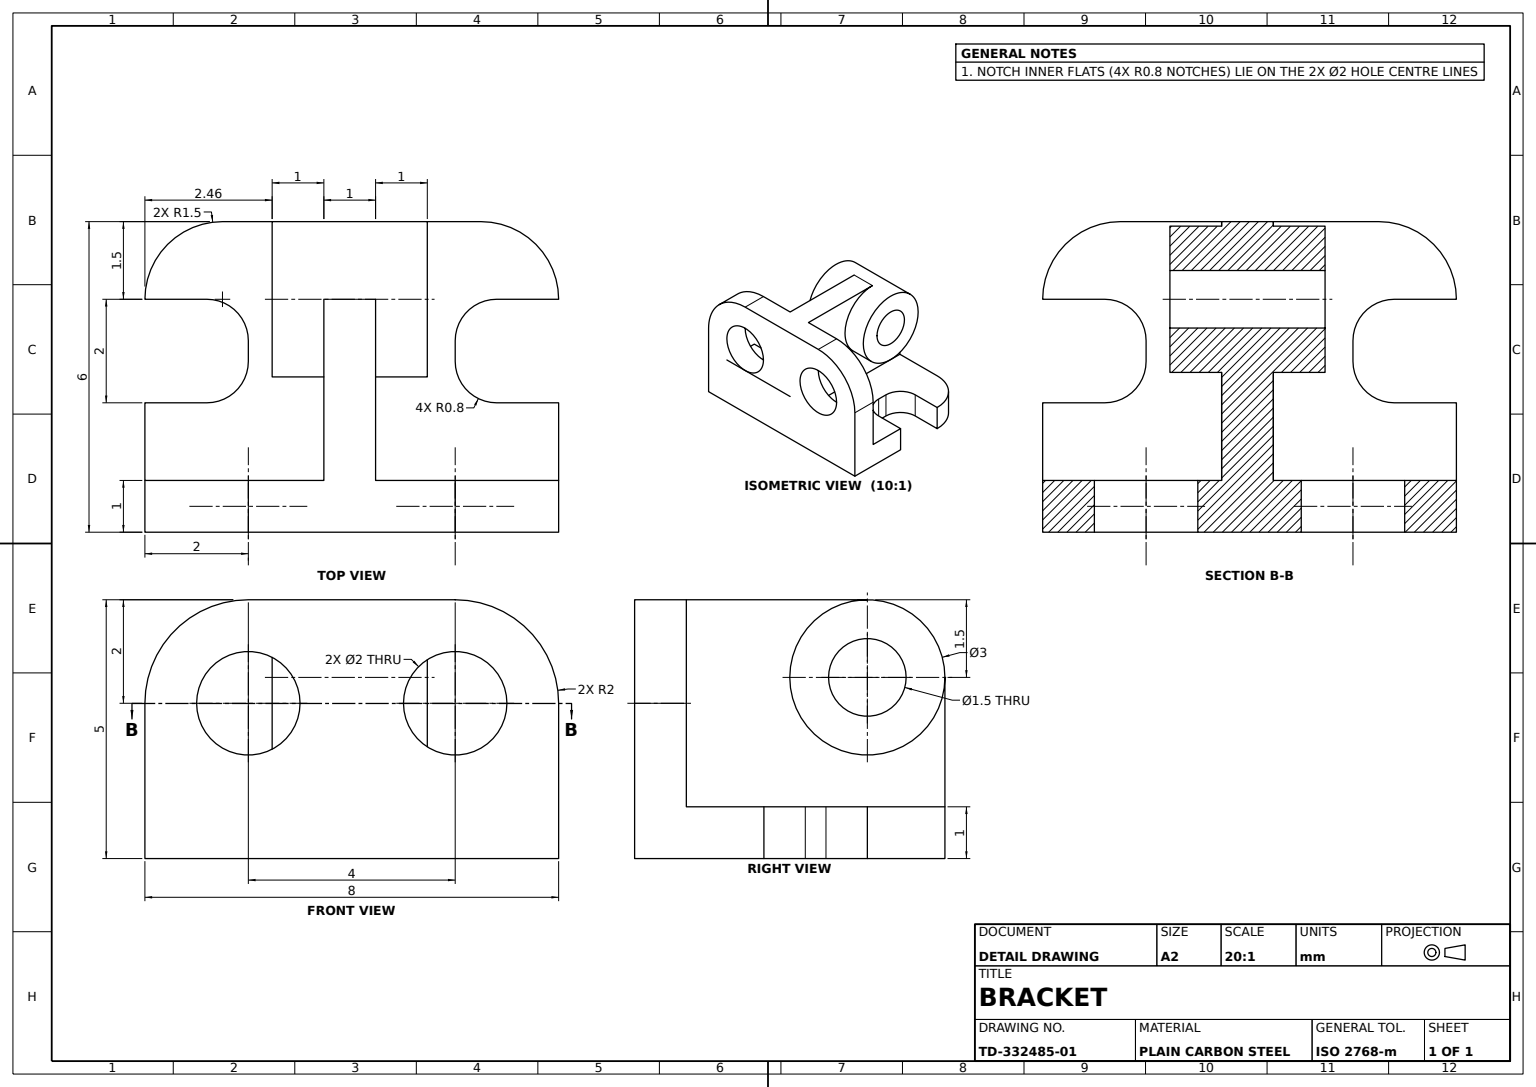
SolidWorks part; units mm, degrees
material "Plain Carbon Steel"
ref_plane "Front Plane" through (0, 0, 0) normal (0, 0, 1) x (1, 0, 0)
ref_plane "Top Plane" through (0, 0, 0) normal (0, 1, 0) x (1, 0, 0)
ref_plane "Right Plane" through (0, 0, 0) normal (1, 0, 0) x (0, 0, -1)
sketch "Base Plate Sketch" plane through (0, 0, 0) normal (0, 1, 0) x (1, 0, 0)
  line L0 (-4, 1.5) -> (-2.8, 1.5)
  line L1 (-4, -3) -> (4, -3)
  line L2 (-4, -3) -> (-4, -0.5)
  line L3 (-2.5, 3) -> (2.5, 3)
  line L4 (4, -3) -> (4, -0.5)
  line L5 (-4, -3) -> (4, 3) construction
  line L6 (-4, 3) -> (4, -3) construction
  line L7 (-2, 0.7) -> (-2, 0.3)
  line L8 (-2.8, -0.5) -> (-4, -0.5)
  line L9 (0, -3) -> (0, 3) construction
  line L10 (2.8, -0.5) -> (4, -0.5)
  line L11 (2, 0.7) -> (2, 0.3)
  line L12 (4, 1.5) -> (2.8, 1.5)
  arc A0 (2.5, 3) -> (4, 1.5) centre (2.5, 1.5) cw
  arc A1 (-2.5, 3) -> (-4, 1.5) centre (-2.5, 1.5) ccw
  arc A2 (-2, 0.3) -> (-2.8, -0.5) centre (-2.8, 0.3) cw
  arc A3 (-2, 0.7) -> (-2.8, 1.5) centre (-2.8, 0.7) ccw
  arc A4 (2, 0.3) -> (2.8, -0.5) centre (2.8, 0.3) ccw
  arc A5 (2, 0.7) -> (2.8, 1.5) centre (2.8, 0.7) cw
  point P0 (0, 0)
  point P19 (-2, 1.5)
  dimension "D3" = 1.5
  dimension "D5" = 0.8
  dimension "D1" = 6
  dimension "D2" = 8
  dimension "D4" = 2
extrude "Base Plate" add sketch "Base Plate Sketch" along normal blind 1
sketch "Upright Plate Sketch" plane through (0, 0, 3) normal (0, 0, 1) x (1, 0, 0)
  line L0 (-4, 0) -> (4, 0)
  line L1 (-4, 0) -> (-4, 3)
  line L2 (4, 0) -> (4, 3)
  line L3 (-2, 5) -> (2, 5)
  arc A0 (-2, 5) -> (-4, 3) centre (-2, 3) ccw
  arc A1 (2, 5) -> (4, 3) centre (2, 3) cw
  circle A2 centre (-2, 3) radius 1
  circle A3 centre (2, 3) radius 1
  point P4 (-4, 5)
  dimension "D2" = 2
  dimension "D3" = 2
  dimension "D4" = 2
  dimension "D1" = 5
  dimension "D5" = 3
  dimension "D6" = 4
extrude "Upright Plate" add sketch "Upright Plate Sketch" against normal blind 1
sketch "Rib Direction Line" plane through (0, 1, 0) normal (0, 1, 0) x (1, 0, 0)
  line L1 (4, -2) -> (4, -0.5) construction
  line L16 (-0.5395, -2) -> (0.4605, -2)
  line L19 (4, -2) -> (-4, -2) construction
  point P2 (-0.0395, -2)
  dimension "D1" = 3.5395
  dimension "D2" = 4.0395
sketch "Rib Sketch" plane through (0, 0, 2) normal (0, 0, -1) x (-1, 0, 0)
  line L1 (-4, 1) -> (4, 1) construction
  line L2 (-2, 5) -> (2, 5) construction
  line L3 (-0.4605, 5) -> (0.5395, 5)
  line L4 (0.5395, 5) -> (0.5395, 1)
  line L5 (0.5395, 1) -> (-0.4605, 1)
  line L6 (-0.4605, 1) -> (-0.4605, 5)
  point P0 (0.0395, 1)
  point P9 (0.0395, 5)
  dimension "D1" = 1
  dimension "D2" = 4
extrude "Rib" add sketch "Rib Sketch" along normal blind 5
sketch "Pivot Hub Sketch" plane through (0.4605, 0, 0) normal (1, 0, 0) x (0, 0, -1)
  line L0 (3, 5) -> (-2, 5) construction
  line L1 (3, 5) -> (3, 1) construction
  line L2 (-2, 5) -> (-2, 1) construction
  circle A0 centre (1.5, 3.5) radius 1.5
  dimension "D1" = 1.5
  dimension "D2" = 3.5
extrude "Pivot Hub" add sketch "Pivot Hub Sketch" along normal blind 1 and the other way blind 2
sketch "Hub Bore Sketch" plane through (1.4605, 0, 0) normal (1, 0, 0) x (0, 0, -1)
  circle A0 centre (1.5, 3.5) radius 0.75
  circle A1 centre (1.5, 3.5) radius 1.5 construction
  dimension "D1" = 1.5
  dimension "D2" = 1.5
extrude "Hub Bore" cut sketch "Hub Bore Sketch" against normal blind 3
sketch "Slot Cut Sketch" plane through (0.4605, 0, 0) normal (1, 0, 0) x (0, 0, -1)
  line L0 (1.5, 5) -> (3, 5)
  line L1 (3, 5) -> (1.5, 5) construction
  line L2 (3, 5) -> (3, 3.5) construction
  line L3 (3, 5) -> (3, 3.5)
  arc A0 (3, 3.5) -> (1.5, 5) centre (1.5, 3.5) ccw
extrude "Slot Cut" cut sketch "Slot Cut Sketch" against normal blind 3
